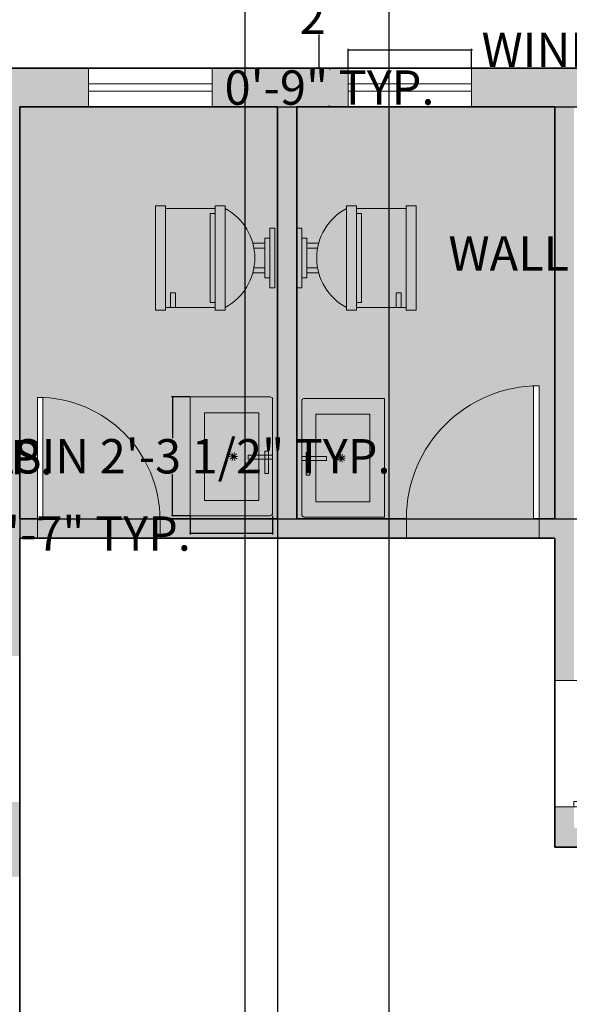
# Model space of a CAD drawing. Units: inches. Extents: x 853 to 1550, y 485 to 1596.
# Tile 15 of 18: x 1139 to 1267, y 1208 to 1437. Entities that reach past the tile are written whole.
import ezdxf

# ---------------------------------------------------------------- set-up
doc = ezdxf.new("R2010")
doc.units = ezdxf.units.IN
doc.header["$MEASUREMENT"] = 0
for name, color, linetype, lineweight in [('A-ANNO-DIMS', 2, 'Continuous', 18), ('A-DOOR', 4, 'Continuous', 18), ('A-FLOR-FIXT', 8, 'Continuous', 18), ('A-WALL-PATT', 250, 'Continuous', 13), ('walls', 250, 'Continuous', 35), ('windows', 4, 'Continuous', 18)]:
    doc.layers.add(name, color=color, linetype=linetype, lineweight=lineweight)
doc.layers.add('A-FIXT-PATT', color=9, linetype='Continuous', lineweight=13, true_color=0xc7c8ca)
doc.layers.add('A-FLOR-TILE-PATT', color=141, linetype='Continuous', lineweight=13, true_color=0xadddf7)
doc.styles.get("Standard").update_dxf_attribs({"font": 'arial.ttf'})
doc.dimstyles.get("Standard").update_dxf_attribs({"dimtxt": 8, "dimasz": 0.18, "dimexe": 0.18, "dimexo": 0.0625, "dimgap": 0.09, "dimtad": 0, "dimtih": 1, "dimtoh": 1, "dimzin": 0, "dimdsep": 46, "dimlunit": 3, "dimtxsty": 'Standard', "dimcen": 0.09, "dimadec": 0, "dimazin": 0, "dimtfac": 1, "dimtofl": 0, "dimtmove": 0, "dimatfit": 3, "dimfxl": 1, "dimtolj": 1, "dimtzin": 0, "dimarcsym": 0})

# ---------------------------------------------------------------- blocks, each defined once
blk = doc.blocks.new('*U10')
for p, q in [((0, 0), (0, -6)), ((40, 0), (40, -6))]:
    blk.add_line(p, q)
blk.add_lwpolyline([(0, 0), (0, 40), (1.75, 40), (1.75, 0)], close=True)
blk.add_arc((0, 0), 40, 0, 90)
blk = doc.blocks.new('*U5')
for p, q in [((-10, 22), (-10, 12)), ((10, 12), (10, 22)), ((-10, 21), (-7, 21)), ((-7, 20), (-10, 20)), ((-7, 21), (-7, 20)), ((10.5, 12), (-10.5, 12)), ((-10.5, 10), (-10.5, 12)), ((9, 13), (-9, 13)), ((-9, 13), (-9, 12)), ((9, 12), (9, 13)), ((10.5, 12), (10.5, 10)), ((10.5, 10), (-10.5, 10)), ((-3, 4.4065), (-3, 2)), ((-2, 2), (-2, 4.1658)), ((2, 4.1658), (2, 2)), ((3, 2), (3, 4.4065)), ((4, 2), (-4, 2)), ((-4, 2), (-4, 1)), ((4, 1), (4, 2))]:
    blk.add_line(p, q)
for points in [[(10.5, 22), (10.5, 24), (-10.5, 24), (-10.5, 22)], [(6, 0), (6, 1), (-6, 1), (-6, 0)]]:
    blk.add_lwpolyline(points, close=True)
blk.add_arc((0, 15.3333), 11.3333, 208.0725, 331.9275)
blk = doc.blocks.new('*D19')
at = {"layer": 'A-ANNO-DIMS', "color": 0, "lineweight": -2, "transparency": 16777216}
for p, q in [((1209.13, 1449.95), (1209.13, 1442.24)), ((1209.19, 1450.13), (1209.31, 1450.13)), ((1209.13, 1426.31), (1209.13, 1434.02)), ((1209.19, 1426.13), (1209.31, 1426.13))]:
    blk.add_line(p, q, dxfattribs=at)
at = {"layer": 'A-ANNO-DIMS', "color": 0, "transparency": 16777216}
for points in [[(1209.1, 1449.95), (1209.16, 1449.95), (1209.13, 1450.13)], [(1209.1, 1426.31), (1209.16, 1426.31), (1209.13, 1426.13)]]:
    blk.add_solid(points, dxfattribs=at)
at = {"layer": 'Defpoints', "color": 0, "transparency": 16777216}
for p in [(1209.13, 1450.13), (1209.13, 1426.13), (1209.13, 1426.13)]:
    blk.add_point(p, dxfattribs=at)
at = {"layer": 'A-ANNO-DIMS', "color": 0, "transparency": 16777216, "insert": (1209.13, 1438.13), "char_height": 8, "attachment_point": 5}
blk.add_mtext("\\A1;2'", dxfattribs=at)
blk = doc.blocks.new('BASIN-RECT-WITH-MIXER')
for p, q in [((0, 3.21), (0, 19.18)), ((0, 19.18), (27.7, 19.18)), ((27.7, 19.18), (27.7, 0.61)), ((3.57, 3.21), (3.57, 15.84)), ((24, 15.84), (24, 3.21)), ((13.79, 9.14), (12.86, 9.39)), ((13.79, 9.14), (13.18, 9.89)), ((13.79, 9.14), (13.74, 10.1)), ((13.79, 9.14), (14.31, 9.95)), ((13.79, 9.14), (14.69, 9.48)), ((13.79, 9.14), (12.89, 8.8)), ((13.79, 9.14), (13.26, 8.33)), ((13.79, 9.14), (14.39, 8.39)), ((13.79, 9.14), (13.83, 8.18)), ((13.79, 9.14), (14.72, 8.89)), ((13.18, 5.79), (13.18, 0)), ((14.12, 5.69), (13.18, 5.69)), ((14.12, 0), (14.12, 5.69)), ((0, 0.61), (0, 3.21)), ((24, 3.21), (3.57, 3.21)), ((27.28, 0), (0.42, 0)), ((15.05, 1.84), (9.82, 1.84)), ((9.82, 1.84), (9.82, 0.98)), ((9.82, 0.98), (11.8, 0.98)), ((11.8, 0.98), (15.05, 0.98)), ((15.05, 0.98), (15.05, 1.84))]:
    blk.add_line(p, q)
for centre, start, end in [((0.76, 0.68), 185.6886, 243.8456), ((26.94, 0.68), 296.1544, 354.3114)]:
    blk.add_arc(centre, 0.761, start, end)
blk = doc.blocks.new('WIN-BATH-29IN')
for p, q in [((0, 9), (0, 0)), ((28.75, 9), (0, 9)), ((0, 9), (0, 6.23)), ((28.75, 0), (28.75, 9)), ((0, 5.38), (28.75, 5.38)), ((28.75, 6.23), (28.75, 4.5)), ((28.75, 3.66), (0, 3.66)), ((0, 0), (28.75, 0))]:
    blk.add_line(p, q)
blk = doc.blocks.new('*D37')
at = {"layer": 'A-ANNO-DIMS', "color": 0, "lineweight": -2, "transparency": 16777216}
for p, q in [((1085.15, 1385.39), (1100.23, 1385.39)), ((1100.05, 1385.21), (1100.05, 1339.74)), ((1100.05, 1285.81), (1100.05, 1331.29)), ((1085.15, 1285.63), (1100.23, 1285.63))]:
    blk.add_line(p, q, dxfattribs=at)
at = {"layer": 'A-ANNO-DIMS', "color": 0, "transparency": 16777216}
for points in [[(1100.02, 1385.21), (1100.08, 1385.21), (1100.05, 1385.39)], [(1100.02, 1285.81), (1100.08, 1285.81), (1100.05, 1285.63)]]:
    blk.add_solid(points, dxfattribs=at)
at = {"layer": 'Defpoints', "color": 0, "transparency": 16777216}
for p in [(1085.09, 1385.39), (1085.09, 1285.63), (1100.05, 1285.63)]:
    blk.add_point(p, dxfattribs=at)
at = {"layer": 'A-ANNO-DIMS', "color": 0, "transparency": 16777216, "insert": (1100.05, 1335.51), "char_height": 8, "attachment_point": 5}
blk.add_mtext('\\A1;BED SET 8\'-4" TYP.', dxfattribs=at)
blk = doc.blocks.new('*D39')
at = {"layer": 'A-ANNO-DIMS', "color": 0, "lineweight": -2, "transparency": 16777216}
for p, q in [((1179.06, 1349.58), (1174.79, 1349.58)), ((1174.97, 1349.4), (1174.97, 1339.96)), ((1174.97, 1322.06), (1174.97, 1331.5)), ((1179.06, 1321.88), (1174.79, 1321.88))]:
    blk.add_line(p, q, dxfattribs=at)
at = {"layer": 'A-ANNO-DIMS', "color": 0, "transparency": 16777216}
for points in [[(1174.94, 1349.4), (1175, 1349.4), (1174.97, 1349.58)], [(1174.94, 1322.06), (1175, 1322.06), (1174.97, 1321.88)]]:
    blk.add_solid(points, dxfattribs=at)
at = {"layer": 'Defpoints', "color": 0, "transparency": 16777216}
for p in [(1174.97, 1349.58), (1179.12, 1349.58), (1179.12, 1321.88)]:
    blk.add_point(p, dxfattribs=at)
at = {"layer": 'A-ANNO-DIMS', "color": 0, "transparency": 16777216, "insert": (1174.97, 1335.73), "char_height": 8, "attachment_point": 5}
blk.add_mtext('\\A1;BASIN 2\'-3 1/2" TYP.', dxfattribs=at)
blk = doc.blocks.new('*D40')
at = {"layer": 'A-ANNO-DIMS', "color": 0, "lineweight": -2, "transparency": 16777216}
for p, q in [((1179.12, 1321.82), (1179.12, 1317.54)), ((1198.3, 1321.82), (1198.3, 1317.54)), ((1179.12, 1317.72), (1178.94, 1317.72)), ((1198.12, 1317.72), (1179.3, 1317.72))]:
    blk.add_line(p, q, dxfattribs=at)
at = {"layer": 'A-ANNO-DIMS', "color": 0, "transparency": 16777216}
for points in [[(1179.3, 1317.75), (1179.3, 1317.69), (1179.12, 1317.72)], [(1198.12, 1317.75), (1198.12, 1317.69), (1198.3, 1317.72)]]:
    blk.add_solid(points, dxfattribs=at)
at = {"layer": 'Defpoints', "color": 0, "transparency": 16777216}
for p in [(1179.12, 1321.88), (1198.3, 1321.88), (1179.12, 1317.72)]:
    blk.add_point(p, dxfattribs=at)
at = {"layer": 'A-ANNO-DIMS', "color": 0, "transparency": 16777216, "insert": (1154.85, 1317.72), "char_height": 8, "attachment_point": 5}
blk.add_mtext('\\A1;1\'-7" TYP.', dxfattribs=at)
blk = doc.blocks.new('*D51')
at = {"layer": 'A-ANNO-DIMS', "color": 0, "lineweight": -2, "transparency": 16777216}
for p, q in [((1215.84, 1426.19), (1215.84, 1430.62)), ((1216.02, 1430.44), (1244.42, 1430.44)), ((1244.6, 1426.19), (1244.6, 1430.62)), ((1244.6, 1430.44), (1244.78, 1430.44))]:
    blk.add_line(p, q, dxfattribs=at)
at = {"layer": 'A-ANNO-DIMS', "color": 0, "transparency": 16777216}
for points in [[(1216.02, 1430.47), (1216.02, 1430.41), (1215.84, 1430.44)], [(1244.42, 1430.47), (1244.42, 1430.41), (1244.6, 1430.44)]]:
    blk.add_solid(points, dxfattribs=at)
at = {"layer": 'Defpoints', "color": 0, "transparency": 16777216}
for p in [(1244.6, 1430.44), (1215.84, 1426.13), (1244.6, 1426.13)]:
    blk.add_point(p, dxfattribs=at)
at = {"layer": 'A-ANNO-DIMS', "color": 0, "transparency": 16777216, "insert": (1295.48, 1430.44), "char_height": 8, "attachment_point": 5}
blk.add_mtext('\\A1;WINDOW 2\'-5" TYP.', dxfattribs=at)
blk = doc.blocks.new('*D52')
at = {"layer": 'A-ANNO-DIMS', "color": 0, "lineweight": -2, "transparency": 16777216}
for p, q in [((1215.78, 1426.13), (1211.35, 1426.13)), ((1211.53, 1425.95), (1211.53, 1425.8)), ((1215.78, 1417.13), (1211.35, 1417.13)), ((1211.53, 1417.31), (1211.53, 1417.45))]:
    blk.add_line(p, q, dxfattribs=at)
at = {"layer": 'A-ANNO-DIMS', "color": 0, "transparency": 16777216}
for points in [[(1211.5, 1425.95), (1211.56, 1425.95), (1211.53, 1426.13)], [(1211.5, 1417.31), (1211.56, 1417.31), (1211.53, 1417.13)]]:
    blk.add_solid(points, dxfattribs=at)
at = {"layer": 'Defpoints', "color": 0, "transparency": 16777216}
for p in [(1211.53, 1426.13), (1215.84, 1426.13), (1215.84, 1417.13)]:
    blk.add_point(p, dxfattribs=at)
at = {"layer": 'A-ANNO-DIMS', "color": 0, "transparency": 16777216, "insert": (1211.53, 1421.63), "char_height": 8, "attachment_point": 5}
blk.add_mtext('\\A1;0\'-9" TYP.', dxfattribs=at)
blk = doc.blocks.new('*D57')
at = {"layer": 'A-ANNO-DIMS', "color": 0, "lineweight": -2, "transparency": 16777216}
for p, q in [((1287.27, 1411.9), (1296.06, 1411.9)), ((1295.88, 1411.72), (1295.88, 1387.16)), ((1295.88, 1354.25), (1295.88, 1378.81)), ((1287.27, 1354.07), (1296.06, 1354.07))]:
    blk.add_line(p, q, dxfattribs=at)
at = {"layer": 'A-ANNO-DIMS', "color": 0, "transparency": 16777216}
for points in [[(1295.85, 1411.72), (1295.91, 1411.72), (1295.88, 1411.9)], [(1295.85, 1354.25), (1295.91, 1354.25), (1295.88, 1354.07)]]:
    blk.add_solid(points, dxfattribs=at)
at = {"layer": 'Defpoints', "color": 0, "transparency": 16777216}
for p in [(1287.21, 1411.9), (1295.88, 1411.9), (1287.21, 1354.07)]:
    blk.add_point(p, dxfattribs=at)
at = {"layer": 'A-ANNO-DIMS', "color": 0, "transparency": 16777216, "insert": (1295.88, 1382.99), "char_height": 8, "attachment_point": 5}
blk.add_mtext('\\A1;WALL UNIT 4\'-10" TYP.', dxfattribs=at)
blk = doc.blocks.new('*D69')
at = {"layer": 'A-ANNO-DIMS', "color": 0, "lineweight": -2, "transparency": 16777216}
for p, q in [((981.94, 1426.19), (981.94, 1584.65)), ((982.12, 1584.47), (1184.11, 1584.47)), ((1413.76, 1584.47), (1211.77, 1584.47)), ((1413.94, 1426.19), (1413.94, 1584.65))]:
    blk.add_line(p, q, dxfattribs=at)
at = {"layer": 'A-ANNO-DIMS', "color": 0, "transparency": 16777216}
for points in [[(982.12, 1584.5), (982.12, 1584.44), (981.94, 1584.47)], [(1413.76, 1584.5), (1413.76, 1584.44), (1413.94, 1584.47)]]:
    blk.add_solid(points, dxfattribs=at)
at = {"layer": 'Defpoints', "color": 0, "transparency": 16777216}
for p in [(1413.94, 1584.47), (981.94, 1426.13), (1413.94, 1426.13)]:
    blk.add_point(p, dxfattribs=at)
at = {"layer": 'A-ANNO-DIMS', "color": 0, "transparency": 16777216, "insert": (1197.94, 1584.47), "char_height": 8, "attachment_point": 5}
blk.add_mtext('\\A1;36\'-0"', dxfattribs=at)
blk = doc.blocks.new('*D72')
at = {"layer": 'A-ANNO-DIMS', "color": 0, "lineweight": -2, "transparency": 16777216}
for p, q in [((1139.44, 1321.07), (1139.44, 497.1)), ((1199.44, 1321.07), (1199.44, 497.1)), ((1139.62, 497.28), (1158.71, 497.28)), ((1199.26, 497.28), (1180.16, 497.28))]:
    blk.add_line(p, q, dxfattribs=at)
at = {"layer": 'A-ANNO-DIMS', "color": 0, "transparency": 16777216}
for points in [[(1139.62, 497.31), (1139.62, 497.25), (1139.44, 497.28)], [(1199.26, 497.31), (1199.26, 497.25), (1199.44, 497.28)]]:
    blk.add_solid(points, dxfattribs=at)
at = {"layer": 'Defpoints', "color": 0, "transparency": 16777216}
for p in [(1139.44, 1321.13), (1199.44, 1321.13), (1199.44, 497.28)]:
    blk.add_point(p, dxfattribs=at)
at = {"layer": 'A-ANNO-DIMS', "color": 0, "transparency": 16777216, "insert": (1169.44, 497.28), "char_height": 8, "attachment_point": 5}
blk.add_mtext('\\A1;5\'-0"', dxfattribs=at)
blk = doc.blocks.new('*D73')
at = {"layer": 'A-ANNO-DIMS', "color": 0, "lineweight": -2, "transparency": 16777216}
for p, q in [((1139.5, 1417.13), (1526.24, 1417.13)), ((1526.06, 1416.95), (1526.06, 1373.3)), ((1526.06, 1321.31), (1526.06, 1364.95)), ((1139.5, 1321.13), (1526.24, 1321.13))]:
    blk.add_line(p, q, dxfattribs=at)
at = {"layer": 'A-ANNO-DIMS', "color": 0, "transparency": 16777216}
for points in [[(1526.03, 1416.95), (1526.09, 1416.95), (1526.06, 1417.13)], [(1526.03, 1321.31), (1526.09, 1321.31), (1526.06, 1321.13)]]:
    blk.add_solid(points, dxfattribs=at)
at = {"layer": 'Defpoints', "color": 0, "transparency": 16777216}
for p in [(1139.44, 1417.13), (1139.44, 1321.13), (1526.06, 1321.13)]:
    blk.add_point(p, dxfattribs=at)
at = {"layer": 'A-ANNO-DIMS', "color": 0, "transparency": 16777216, "insert": (1526.06, 1369.13), "char_height": 8, "attachment_point": 5}
blk.add_mtext('\\A1;8\'-0"', dxfattribs=at)
blk = doc.blocks.new('*D81')
at = {"layer": 'A-ANNO-DIMS', "color": 0, "lineweight": -2, "transparency": 16777216}
for p, q in [((1191.94, 767.69), (1191.94, 1584.65)), ((1192.12, 1584.47), (1225.27, 1584.47)), ((1225.45, 767.69), (1225.45, 1584.65)), ((1225.45, 1584.47), (1225.63, 1584.47))]:
    blk.add_line(p, q, dxfattribs=at)
at = {"layer": 'A-ANNO-DIMS', "color": 0, "transparency": 16777216}
for points in [[(1192.12, 1584.5), (1192.12, 1584.44), (1191.94, 1584.47)], [(1225.27, 1584.5), (1225.27, 1584.44), (1225.45, 1584.47)]]:
    blk.add_solid(points, dxfattribs=at)
at = {"layer": 'Defpoints', "color": 0, "transparency": 16777216}
for p in [(1225.45, 1584.47), (1191.94, 767.63), (1225.45, 767.63)]:
    blk.add_point(p, dxfattribs=at)
at = {"layer": 'A-ANNO-DIMS', "color": 0, "transparency": 16777216, "insert": (1245.74, 1584.47), "char_height": 8, "attachment_point": 5}
blk.add_mtext('\\A1;2\'-9 1/2"', dxfattribs=at)

msp = doc.modelspace()

# ---------------------------------------------------------------- hatches: boundary and pattern name
at = {"layer": 'A-FIXT-PATT'}
h = msp.add_hatch(color=256, dxfattribs=at)
h.dxf.hatch_style = 1
h.paths.add_polyline_path([(1173.359, 1393.472), (1173.359, 1370.37), (1174.514, 1370.37), (1174.514, 1373.835), (1175.669, 1373.835), (1175.669, 1370.37), (1184.91, 1370.37), (1184.91, 1371.525), (1183.755, 1371.525), (1183.755, 1392.316), (1184.91, 1392.316), (1184.91, 1393.472)])
h.paths.add_polyline_path([(1171.049, 1394.049), (1171.049, 1369.792), (1173.359, 1369.792), (1173.359, 1394.049)])
h.paths.add_polyline_path([(1184.91, 1394.049), (1184.91, 1369.792), (1187.22, 1369.792), (1187.22, 1394.049)])
h.paths.add_polyline_path([(1183.755, 1392.316), (1183.755, 1371.525), (1184.91, 1371.525), (1184.91, 1392.316)], flags=17)
h.paths.add_polyline_path([(1187.22, 1393.472), (1187.22, 1370.37, 0.6000022)])
h.paths.add_polyline_path([(1193.945, 1379.61, -0.0226287), (1193.684, 1378.455), (1196.461, 1378.455), (1196.461, 1379.61)])
h.paths.add_polyline_path([(1193.684, 1385.386, -0.0226287), (1193.945, 1384.231), (1196.461, 1384.231), (1196.461, 1385.386)])
h.paths.add_polyline_path([(1196.461, 1386.541), (1196.461, 1377.3), (1197.616, 1377.3), (1197.616, 1386.541)])
h.paths.add_polyline_path([(1197.616, 1388.851), (1197.616, 1374.99), (1198.771, 1374.99), (1198.771, 1388.851)])
h = msp.add_hatch(color=256, dxfattribs=at)
h.dxf.hatch_style = 1
h.paths.add_polyline_path([(1229.349, 1393.474), (1229.349, 1370.372), (1228.194, 1370.372), (1228.194, 1373.837), (1227.039, 1373.837), (1227.039, 1370.372), (1217.798, 1370.372), (1217.798, 1371.527), (1218.953, 1371.527), (1218.953, 1392.319), (1217.798, 1392.319), (1217.798, 1393.474)])
h.paths.add_polyline_path([(1231.659, 1394.051), (1231.659, 1369.794), (1229.349, 1369.794), (1229.349, 1394.051)])
h.paths.add_polyline_path([(1217.798, 1394.051), (1217.798, 1369.794), (1215.488, 1369.794), (1215.488, 1394.051)])
h.paths.add_polyline_path([(1218.953, 1392.319), (1218.953, 1371.527), (1217.798, 1371.527), (1217.798, 1392.319)], flags=17)
h.paths.add_polyline_path([(1215.488, 1393.474), (1215.488, 1370.372, -0.6000022)])
h.paths.add_polyline_path([(1208.763, 1379.613, 0.0226287), (1209.024, 1378.458), (1206.247, 1378.458), (1206.247, 1379.613)])
h.paths.add_polyline_path([(1209.024, 1385.388, 0.0226287), (1208.763, 1384.233), (1206.247, 1384.233), (1206.247, 1385.388)])
h.paths.add_polyline_path([(1206.247, 1386.543), (1206.247, 1377.303), (1205.092, 1377.303), (1205.092, 1386.543)])
h.paths.add_polyline_path([(1205.092, 1388.853), (1205.092, 1374.992), (1203.937, 1374.992), (1203.937, 1388.853)])
h = msp.add_hatch(color=256, dxfattribs=at)
h.dxf.hatch_style = 1
h.paths.add_polyline_path([(1182.467, 1325.447), (1182.467, 1345.883), (1195.095, 1345.883), (1195.095, 1335.997), (1196.466, 1335.997), (1196.466, 1336.932), (1197.325, 1336.932), (1197.325, 1335.997), (1198.303, 1335.997), (1198.303, 1349.154, 0.2593488), (1197.696, 1349.576), (1179.123, 1349.576), (1179.123, 1321.879), (1195.095, 1321.879), (1197.696, 1321.879, 0.2593488), (1198.303, 1322.301), (1198.303, 1335.06), (1197.325, 1335.06), (1197.325, 1333.678), (1197.325, 1331.695), (1196.466, 1331.695), (1196.466, 1335.06), (1195.095, 1335.06), (1195.095, 1325.447)])
h = msp.add_hatch(color=256, dxfattribs=at)
h.dxf.hatch_style = 1
h.paths.add_polyline_path([(1220.947, 1325.094), (1220.947, 1345.531), (1208.319, 1345.531), (1208.319, 1335.644), (1206.948, 1335.644), (1206.948, 1336.579), (1206.089, 1336.579), (1206.089, 1335.644), (1205.111, 1335.644), (1205.111, 1348.801, -0.2593488), (1205.718, 1349.223), (1224.291, 1349.223), (1224.291, 1321.527), (1208.319, 1321.527), (1205.718, 1321.527, -0.2593488), (1205.111, 1321.948), (1205.111, 1334.708), (1206.089, 1334.708), (1206.089, 1333.325), (1206.089, 1331.343), (1206.948, 1331.343), (1206.948, 1334.708), (1208.319, 1334.708), (1208.319, 1325.094)])
h = msp.add_hatch(color=256, dxfattribs=at)
h.dxf.hatch_style = 1
h.paths.add_polyline_path([(1182.467, 1345.883), (1182.467, 1325.447), (1195.095, 1325.447), (1195.095, 1335.06), (1192.617, 1335.06), (1192.617, 1335.997), (1195.095, 1335.997), (1195.095, 1345.883)])
h.paths.add_polyline_path([(1189.164, 1337.69, -1), (1189.164, 1333.639, -1)], flags=16)
h.paths.add_polyline_path([(1189.164, 1336.628, -1), (1189.164, 1334.702, -1)], flags=0)
h.paths.add_polyline_path([(1192.617, 1335.997), (1192.617, 1335.06), (1195.095, 1335.06), (1195.095, 1335.997)], flags=17)
h.paths.add_polyline_path([(1195.095, 1335.997), (1195.095, 1335.06), (1196.466, 1335.06), (1196.466, 1335.997)])
h.paths.add_polyline_path([(1196.466, 1335.997), (1196.466, 1335.06), (1197.325, 1335.06), (1197.325, 1335.997)])
h.paths.add_polyline_path([(1196.466, 1335.06), (1196.466, 1331.695), (1197.325, 1331.695), (1197.325, 1333.678), (1197.325, 1335.06)])
h.paths.add_polyline_path([(1196.466, 1336.932), (1196.466, 1335.997), (1197.325, 1335.997), (1197.325, 1336.932)])
h.paths.add_polyline_path([(1197.325, 1335.997), (1197.325, 1335.06), (1198.303, 1335.06), (1198.303, 1335.997)])
h.paths.add_polyline_path([(1198.303, 1335.997), (1198.303, 1335.06), (1199.416, 1335.06), (1199.416, 1335.997)])
h = msp.add_hatch(color=256, dxfattribs=at)
h.dxf.hatch_style = 1
h.paths.add_polyline_path([(1220.947, 1345.531), (1220.947, 1325.094), (1208.319, 1325.094), (1208.319, 1334.708), (1210.797, 1334.708), (1210.797, 1335.644), (1208.319, 1335.644), (1208.319, 1345.531)])
h.paths.add_polyline_path([(1214.25, 1337.338, 1), (1214.25, 1333.287, 1)], flags=16)
h.paths.add_polyline_path([(1214.25, 1336.275, 1), (1214.25, 1334.35, 1)], flags=0)
h.paths.add_polyline_path([(1210.797, 1335.644), (1210.797, 1334.708), (1208.319, 1334.708), (1208.319, 1335.644)], flags=17)
h.paths.add_polyline_path([(1208.319, 1335.644), (1208.319, 1334.708), (1206.948, 1334.708), (1206.948, 1335.644)])
h.paths.add_polyline_path([(1206.948, 1335.644), (1206.948, 1334.708), (1206.089, 1334.708), (1206.089, 1335.644)])
h.paths.add_polyline_path([(1206.948, 1334.708), (1206.948, 1331.343), (1206.089, 1331.343), (1206.089, 1333.325), (1206.089, 1334.708)])
h.paths.add_polyline_path([(1206.948, 1336.579), (1206.948, 1335.644), (1206.089, 1335.644), (1206.089, 1336.579)])
h.paths.add_polyline_path([(1206.089, 1335.644), (1206.089, 1334.708), (1205.111, 1334.708), (1205.111, 1335.644)])
h.paths.add_polyline_path([(1205.111, 1335.644), (1205.111, 1334.708), (1203.998, 1334.708), (1203.998, 1335.644)])
h = msp.add_hatch(color=256, dxfattribs=at)
h.dxf.hatch_style = 1
h.paths.add_polyline_path([(1189.164, 1333.639, 1), (1189.164, 1337.69, 1)])
h.paths.add_polyline_path([(1189.164, 1336.628, -1), (1189.164, 1334.702, -1)], flags=16)
h = msp.add_hatch(color=256, dxfattribs=at)
h.dxf.hatch_style = 1
h.paths.add_polyline_path([(1214.25, 1333.287, -1), (1214.25, 1337.338, -1)])
h.paths.add_polyline_path([(1214.25, 1336.275, 1), (1214.25, 1334.35, 1)], flags=16)
at = {"layer": 'A-FLOR-TILE-PATT'}
h = msp.add_hatch(dxfattribs=at)
h.set_pattern_fill('ANGLE', color=256, scale=3)
h.set_pattern_definition([(0, (0, 0), (0, 0.825), [0.6, -0.225]), (90, (0, 0), (-0.825, 1e-16), [0.6, -0.225])])
h.paths.add_polyline_path([(1199.437, 1417.129), (1139.437, 1417.129), (1139.437, 1321.129), (1143.553, 1321.129), (1143.553, 1349.459), (1144.802, 1349.459), (1144.802, 1349.432, -0.3992393), (1172.1, 1321.129), (1199.437, 1321.129)])
h.paths.add_polyline_path([(1144.802, 1349.432), (1144.802, 1320.911), (1143.553, 1320.911), (1143.553, 1316.629), (1172.101, 1316.629), (1172.101, 1320.911, 0.4014527)])
h.paths.add_polyline_path([(1263.937, 1417.129), (1203.937, 1417.129), (1203.937, 1321.129), (1229.433, 1321.129), (1229.433, 1321.265, -0.4014527), (1258.988, 1352.143), (1258.988, 1352.172), (1260.34, 1352.172), (1260.34, 1321.129), (1263.937, 1321.129)])
h.paths.add_polyline_path([(1258.988, 1352.143, 0.4027308), (1229.433, 1321.129), (1229.433, 1321.129), (1229.433, 1316.629), (1260.34, 1316.629), (1260.34, 1321.265), (1258.988, 1321.265)])
at = {"layer": 'A-WALL-PATT'}
h = msp.add_hatch(color=256, dxfattribs=at)
h.dxf.hatch_style = 1
h.paths.add_polyline_path([(1139.437, 988.732), (1134.937, 988.732), (1134.937, 830.473), (1139.437, 830.473)])
h.paths.add_polyline_path([(1413.937, 1052.227), (1404.937, 1052.227), (1404.937, 1036.129), (1308.937, 1036.129), (1308.937, 1045.033), (1304.437, 1045.033), (1304.437, 1030.033), (1308.937, 1030.033), (1308.937, 1031.629), (1404.937, 1031.629), (1404.937, 863.629), (1365.241, 863.629), (1365.241, 854.629), (1413.937, 854.629)])
h.paths.add_polyline_path([(1413.937, 1133.918), (1404.937, 1133.918), (1404.937, 1100.629), (1304.437, 1100.629), (1304.437, 1078.26), (1308.937, 1078.26), (1308.937, 1096.129), (1404.937, 1096.129), (1404.937, 1084.233), (1407.946, 1084.233), (1413.937, 1084.233)])
h.paths.add_polyline_path([(1268.437, 1417.129), (1288.974, 1417.129), (1288.974, 1426.129), (1244.597, 1426.129), (1244.597, 1417.129), (1263.937, 1417.129), (1263.937, 1321.129), (1260.34, 1321.129), (1260.34, 1316.629), (1263.937, 1316.629), (1263.937, 1283.505), (1268.437, 1283.505)])
h.paths.add_polyline_path([(1413.937, 1426.129), (1360.402, 1426.129), (1360.402, 1417.129), (1404.937, 1417.129), (1404.937, 1249.129), (1268.437, 1249.129), (1268.437, 1254.041), (1268.357, 1254.041), (1263.937, 1254.041), (1263.937, 1244.629), (1404.937, 1244.629), (1404.937, 1228.163), (1413.937, 1228.163)])
h.paths.add_polyline_path([(1215.842, 1426.129), (1184.201, 1426.129), (1184.201, 1417.129), (1199.437, 1417.129), (1199.437, 1321.129), (1172.101, 1321.129), (1172.101, 1316.629), (1229.433, 1316.629), (1229.433, 1321.129), (1203.937, 1321.129), (1203.937, 1417.129), (1215.842, 1417.129)])
h.paths.add_polyline_path([(1139.437, 1417.129), (1155.446, 1417.129), (1155.446, 1426.129), (1091.831, 1426.129), (1091.831, 1417.129), (1134.937, 1417.129), (1134.937, 1289.22), (1139.437, 1289.22), (1139.437, 1316.629), (1143.553, 1316.629), (1143.553, 1321.129), (1139.437, 1321.129)])
h.paths.add_polyline_path([(1139.437, 1255.161), (1134.937, 1255.161), (1134.937, 1249.129), (990.937, 1249.129), (990.937, 1417.129), (1020.402, 1417.129), (1020.402, 1426.129), (981.937, 1426.129), (981.937, 1205.535), (984.477, 1205.535), (990.937, 1205.535), (990.937, 1244.629), (1134.937, 1244.629), (1134.937, 1237.775), (1139.437, 1237.775)])

# ---------------------------------------------------------------- linework, layer by layer
at = {"layer": 'A-FLOR-FIXT'}
for p, q in [((1182.467, 1325.447), (1182.467, 1345.883)), ((1220.947, 1325.094), (1220.947, 1345.531))]:
    msp.add_line(p, q, dxfattribs=at)
at = {"layer": 'walls'}
for p, q in [((981.937, 1426.129), (1413.937, 1426.129)), ((1139.437, 1321.129), (1139.437, 1417.129)), ((1139.437, 1417.129), (1199.437, 1417.129)), ((1199.437, 1321.129), (1199.437, 1417.129)), ((1203.937, 1321.129), (1203.937, 1417.129)), ((1203.937, 1417.129), (1263.937, 1417.129)), ((1263.937, 1321.129), (1263.937, 1417.129)), ((1139.437, 1321.129), (1143.553, 1321.129)), ((1172.1, 1321.129), (1199.437, 1321.129)), ((1203.937, 1321.129), (1229.433, 1321.129)), ((1260.34, 1321.129), (1263.937, 1321.129)), ((1139.437, 1316.629), (1263.937, 1316.629)), ((1139.437, 1072.129), (1139.437, 1316.629)), ((1263.937, 1244.629), (1263.937, 1316.629)), ((1263.937, 1244.629), (1404.937, 1244.629))]:
    msp.add_line(p, q, dxfattribs=at)

# ---------------------------------------------------------------- block references
at = {"layer": 'A-DOOR'}
for p, xscale, yscale, zscale in [((1260.34, 1321.265), -0.7726693254368758, 0.7726693254368758, 0.7726693254368758), ((1143.553, 1320.911), 0.713693331572247, 0.713693331572247, 0.713693331572247)]:
    msp.add_blockref('*U10', p, dxfattribs=dict(at, xscale=xscale, yscale=yscale, zscale=zscale))
at = {"layer": 'A-DOOR', "xscale": -0.7365814007727343, "yscale": 0.7365814007727343, "zscale": 0.7365814007727343, "rotation": 270}
msp.add_blockref('*U10', (1268.357, 1254.041), dxfattribs=at)
at = {"layer": 'A-FLOR-FIXT', "yscale": 1.155096372646877, "zscale": 1.155096372646877}
for p, xscale, rotation in [((1198.771, 1381.921), 1.155096372646877, 90.00000000000003), ((1203.937, 1381.923), -1.155096372646877, 270)]:
    msp.add_blockref('*U5', p, dxfattribs=dict(at, xscale=xscale, rotation=rotation))
at = {"layer": 'A-FLOR-FIXT', "rotation": 90.00000000000087}
msp.add_blockref('BASIN-RECT-WITH-MIXER', (1198.303, 1321.879), dxfattribs=at)
at = {"layer": 'A-FLOR-FIXT', "extrusion": (0, 0, -1), "zscale": -1, "rotation": 89.99999999999838}
msp.add_blockref('BASIN-RECT-WITH-MIXER', (-1205.111, 1321.526), dxfattribs=at)
at = {"layer": 'windows'}
for p in [(1155.446, 1417.129), (1215.842, 1417.129)]:
    msp.add_blockref('WIN-BATH-29IN', p, dxfattribs=at)

# ---------------------------------------------------------------- dimensions: what is measured, and where the dimension line sits
at = {"layer": 'A-ANNO-DIMS'}
for base, p1, p2, picture, middle in [((1225.453, 1584.468), (1191.938, 767.629), (1225.453, 767.629), '*D81', (1245.744, 1584.468)), ((1413.937, 1584.468), (981.937, 1426.129), (1413.937, 1426.129), '*D69', (1197.937, 1584.468)), ((1199.437, 497.279), (1139.437, 1321.129), (1199.437, 1321.129), '*D72', (1169.437, 497.279))]:
    dim = msp.add_linear_dim(base=base, p1=p1, p2=p2, dimstyle='Standard', override={"dimdec": 1, "dimlfac": 1, "dimrnd": 0, "dimzin": 1, "dimdsep": 46, "dimlunit": 4, "dimfrac": 2}, dxfattribs=at)
    dim.commit()
    dim.dimension.update_dxf_attribs({"geometry": picture, "text_midpoint": middle})
for base, p1, p2, override, picture, middle in [((1209.126, 1426.129), (1209.126, 1450.129), (1209.126, 1426.129), {"dimclrd": 0, "dimclre": 0, "dimclrt": 0}, '*D19', (1209.126, 1438.129)), ((1526.064, 1321.129), (1139.437, 1417.129), (1139.437, 1321.129), {"dimdec": 1, "dimlfac": 1, "dimrnd": 0, "dimzin": 1, "dimdsep": 46, "dimlunit": 4, "dimfrac": 2}, '*D73', (1526.064, 1369.129))]:
    dim = msp.add_linear_dim(base=base, p1=p1, p2=p2, angle=90, dimstyle='Standard', override=override, dxfattribs=at)
    dim.commit()
    dim.dimension.update_dxf_attribs({"geometry": picture, "text_midpoint": middle})
dim = msp.add_linear_dim(base=(1244.597, 1430.443), p1=(1215.842, 1426.129), p2=(1244.597, 1426.129), text='WINDOW <> TYP.', dimstyle='Standard', override={"dimdec": 1, "dimlfac": 1, "dimrnd": 0, "dimzin": 1, "dimdsep": 46, "dimlunit": 4, "dimfrac": 2}, dxfattribs=at)
dim.commit()
dim.dimension.update_dxf_attribs({"geometry": '*D51', "text_midpoint": (1295.484, 1430.443)})
for base, p1, p2, angle, text, picture, middle in [((1211.529, 1426.129), (1215.842, 1417.129), (1215.842, 1426.129), 90, '<> TYP.', '*D52', (1211.529, 1421.629)), ((1295.88, 1411.904), (1287.205, 1354.07), (1287.205, 1411.904), 90, 'WALL UNIT <> TYP.', '*D57', (1295.88, 1382.987)), ((1100.052, 1285.631), (1085.088, 1385.394), (1085.088, 1285.631), 270, 'BED SET <> TYP.', '*D37', (1100.052, 1335.512)), ((1174.969, 1349.576), (1179.123, 1321.879), (1179.123, 1349.576), 90, 'BASIN <> TYP.', '*D39', (1174.969, 1335.727)), ((1179.123, 1317.724), (1198.303, 1321.879), (1179.123, 1321.879), 180, '<> TYP.', '*D40', (1154.848, 1317.724))]:
    dim = msp.add_linear_dim(base=base, p1=p1, p2=p2, angle=angle, text=text, dimstyle='Standard', override={"dimdec": 1, "dimlfac": 1, "dimrnd": 0, "dimzin": 1, "dimdsep": 46, "dimlunit": 4, "dimfrac": 2}, dxfattribs=at)
    dim.commit()
    dim.dimension.update_dxf_attribs({"geometry": picture, "text_midpoint": middle})

doc.saveas('drawing.dxf')
